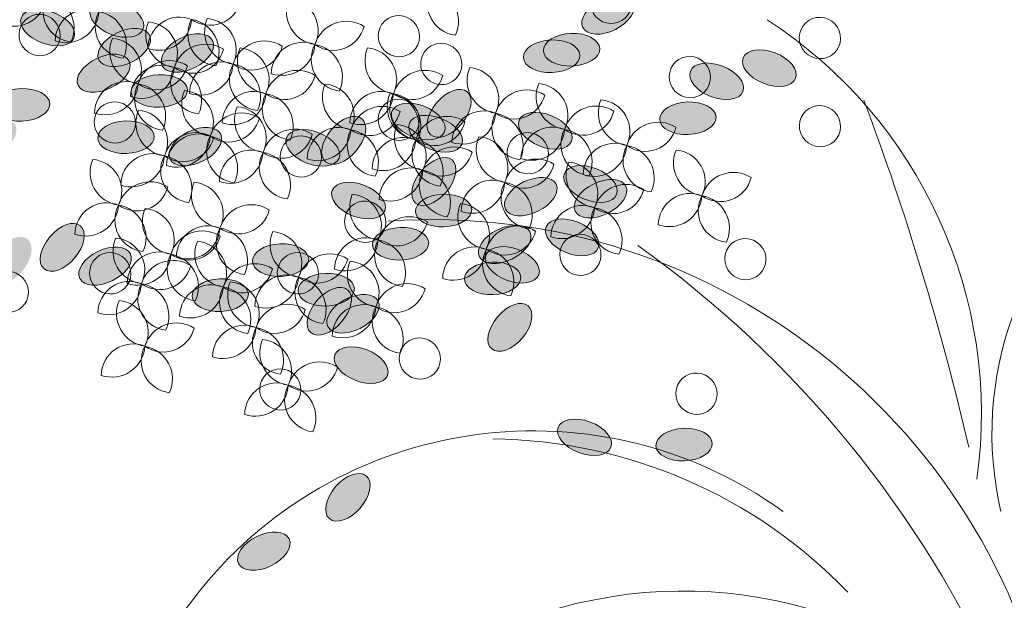
# Model space of a CAD drawing. Units: millimetres. Extents: x 595116 to 630915, y 909473 to 920225.
# Tile 13 of 134: x 629511 to 629534, y 919176 to 919190. Entities that reach past the tile are written whole.
import ezdxf

# ---------------------------------------------------------------- set-up
doc = ezdxf.new("R2010")
doc.units = ezdxf.units.MM
doc.layers.add('Dimension', color=3, linetype='Continuous', lineweight=18)
doc.layers.add('L-PLNT', color=85, linetype='Continuous', lineweight=13)
doc.styles.get("Standard").update_dxf_attribs({"font": 'arial.ttf'})
doc.dimstyles.new('ISO-25', dxfattribs={"dimtxt": 9, "dimasz": 6, "dimexe": 1.25, "dimexo": 0.625, "dimtad": 1, "dimlunit": 4, "dimtxsty": 'Standard', "dimcen": 2.5, "dimadec": 0, "dimazin": 0, "dimtfac": 1, "dimtmove": 0, "dimatfit": 3, "dimfxl": 1, "dimarcsym": 0})

# ---------------------------------------------------------------- blocks, each defined once
blk = doc.blocks.new('tree')
for centre, radius, start, end in [((629595.141, 919296.95), 5.184, 352.032, 57.0714), ((629604.232, 919296.737), 3.791, 61.1347, 193.108), ((629569.835, 919289.496), 31.168, 13.149, 20.5076), ((629594.259, 919292.132), 6.965, 7.4001, 94.0059), ((629589.446, 919288.922), 12.167, 24.2477, 54.3726), ((629595.377, 919292.044), 4.722, 54.2484, 144.2167), ((629594.88, 919291.171), 5.506, 43.8672, 89.4805), ((629597.025, 919289.989), 5.01, 36.0581, 170.6542)]:
    blk.add_arc(centre, radius, start, end)
blk = doc.blocks.new('A$C77972600')
h = blk.add_hatch(color=256)
edge = h.paths.add_edge_path()
edge.add_ellipse((3.0705, 5.8276), major_axis=(-0.1731, 0.0699), ratio=0.578492, start_angle=0, end_angle=360)
edge = h.paths.add_edge_path()
edge.add_ellipse((4.0989, 6.0027), major_axis=(-0.1319, 0.1321), ratio=0.578492, start_angle=0, end_angle=360)
edge = h.paths.add_edge_path()
edge.add_ellipse((4.5318, 6.7683), major_axis=(-0.1688, -0.0798), ratio=0.578492, start_angle=0, end_angle=360)
edge = h.paths.add_edge_path()
edge.add_ellipse((5.185, 6.8705), major_axis=(-0.1865, -0.0073), ratio=0.578492, start_angle=0, end_angle=360)
edge = h.paths.add_edge_path()
edge.add_ellipse((4.6885, 3.4464), major_axis=(-0.1865, -0.0073), ratio=0.578492, start_angle=0, end_angle=360)
edge = h.paths.add_edge_path()
edge.add_ellipse((4.5217, 4.2367), major_axis=(-0.1865, -0.0073), ratio=0.578492, start_angle=0, end_angle=360)
edge = h.paths.add_edge_path()
edge.add_ellipse((4.9166, 3.9946), major_axis=(-0.1731, 0.0699), ratio=0.578492, start_angle=0, end_angle=360)
edge = h.paths.add_edge_path()
edge.add_ellipse((3.6759, 4.9988), major_axis=(-0.1319, 0.1321), ratio=0.578492, start_angle=0, end_angle=360)
edge = h.paths.add_edge_path()
edge.add_ellipse((3.1035, 4.6784), major_axis=(-0.1319, 0.1321), ratio=0.578492, start_angle=0, end_angle=360)
edge = h.paths.add_edge_path()
edge.add_ellipse((3.8133, 4.5577), major_axis=(-0.1319, 0.1321), ratio=0.578492, start_angle=0, end_angle=360)
edge = h.paths.add_edge_path()
edge.add_ellipse((2.2042, 5.6327), major_axis=(-0.1865, -0.0073), ratio=0.578492, start_angle=0, end_angle=360)
edge = h.paths.add_edge_path()
edge.add_ellipse((2.9066, 5.6543), major_axis=(-0.1865, -0.0073), ratio=0.578492, start_angle=0, end_angle=360)
edge = h.paths.add_edge_path()
edge.add_ellipse((2.6215, 5.4344), major_axis=(-0.1865, -0.0073), ratio=0.578492, start_angle=0, end_angle=360)
edge = h.paths.add_edge_path()
edge.add_ellipse((2.1195, 4.0174), major_axis=(-0.1731, 0.0699), ratio=0.578492, start_angle=0, end_angle=360)
edge = h.paths.add_edge_path()
edge.add_ellipse((4.1491, 5.5914), major_axis=(-0.1688, -0.0798), ratio=0.578492, start_angle=0, end_angle=360)
edge = h.paths.add_edge_path()
edge.add_ellipse((1.9571, 3.173), major_axis=(-0.1865, -0.0073), ratio=0.578492, start_angle=0, end_angle=360)
edge = h.paths.add_edge_path()
edge.add_ellipse((1.589, 3.2907), major_axis=(-0.1688, -0.0798), ratio=0.578492, start_angle=0, end_angle=360)
edge = h.paths.add_edge_path()
edge.add_ellipse((1.045, 3.0811), major_axis=(-0.1865, -0.0073), ratio=0.578492, start_angle=0, end_angle=360)
edge = h.paths.add_edge_path()
edge.add_ellipse((1.2104, 3.7739), major_axis=(-0.1688, -0.0798), ratio=0.578492, start_angle=0, end_angle=360)
edge = h.paths.add_edge_path()
edge.add_ellipse((1.6721, 3.755), major_axis=(-0.1688, -0.0798), ratio=0.578492, start_angle=0, end_angle=360)
edge = h.paths.add_edge_path()
edge.add_ellipse((0.772, 4.473), major_axis=(-0.1731, 0.0699), ratio=0.578492, start_angle=0, end_angle=360)
edge = h.paths.add_edge_path()
edge.add_ellipse((0.8326, 5.2916), major_axis=(-0.1319, 0.1321), ratio=0.578492, start_angle=0, end_angle=360)
edge = h.paths.add_edge_path()
edge.add_ellipse((1.1875, 5.2313), major_axis=(-0.1319, 0.1321), ratio=0.578492, start_angle=0, end_angle=360)
edge = h.paths.add_edge_path()
edge.add_ellipse((5.3876, 4.7197), major_axis=(-0.1865, -0.0073), ratio=0.578492, start_angle=0, end_angle=360)
edge = h.paths.add_edge_path()
edge.add_ellipse((3.5552, 2.162), major_axis=(-0.1865, -0.0073), ratio=0.578492, start_angle=0, end_angle=360)
edge = h.paths.add_edge_path()
edge.add_ellipse((3.8402, 2.3819), major_axis=(-0.1865, -0.0073), ratio=0.578492, start_angle=0, end_angle=360)
edge = h.paths.add_edge_path()
edge.add_ellipse((4.692, 2.204), major_axis=(-0.1731, 0.0699), ratio=0.578492, start_angle=0, end_angle=360)
edge = h.paths.add_edge_path()
edge.add_ellipse((4.514, 2.9096), major_axis=(-0.1731, 0.0699), ratio=0.578492, start_angle=0, end_angle=360)
edge = h.paths.add_edge_path()
edge.add_ellipse((4.8133, 2.5575), major_axis=(-0.1731, 0.0699), ratio=0.578492, start_angle=0, end_angle=360)
edge = h.paths.add_edge_path()
edge.add_ellipse((3.7876, 2.8899), major_axis=(-0.1731, 0.0699), ratio=0.578492, start_angle=0, end_angle=360)
h = blk.add_hatch(color=256)
edge = h.paths.add_edge_path()
edge.add_ellipse((3.2403, 1.6985), major_axis=(-0.1668, -0.0838), ratio=0.578492, start_angle=0, end_angle=360, ccw=False)
edge = h.paths.add_edge_path()
edge.add_ellipse((4.2796, 1.6084), major_axis=(-0.1206, -0.1425), ratio=0.578492, start_angle=0, end_angle=360, ccw=False)
edge = h.paths.add_edge_path()
edge.add_ellipse((4.7739, 0.881), major_axis=(-0.1747, 0.0657), ratio=0.578492, start_angle=0, end_angle=360, ccw=False)
edge = h.paths.add_edge_path()
edge.add_ellipse((5.4333, 0.8328), major_axis=(-0.1865, -0.008), ratio=0.578492, start_angle=0, end_angle=360, ccw=False)
edge = h.paths.add_edge_path()
edge.add_ellipse((4.6573, 4.2045), major_axis=(-0.1865, -0.008), ratio=0.578492, start_angle=0, end_angle=360, ccw=False)
edge = h.paths.add_edge_path()
edge.add_ellipse((4.556, 3.4032), major_axis=(-0.1865, -0.008), ratio=0.578492, start_angle=0, end_angle=360, ccw=False)
edge = h.paths.add_edge_path()
edge.add_ellipse((4.9297, 3.677), major_axis=(-0.1668, -0.0838), ratio=0.578492, start_angle=0, end_angle=360, ccw=False)
edge = h.paths.add_edge_path()
edge.add_ellipse((3.7756, 2.5742), major_axis=(-0.1206, -0.1425), ratio=0.578492, start_angle=0, end_angle=360, ccw=False)
edge = h.paths.add_edge_path()
edge.add_ellipse((3.1788, 2.8466), major_axis=(-0.1206, -0.1425), ratio=0.578492, start_angle=0, end_angle=360, ccw=False)
edge = h.paths.add_edge_path()
edge.add_ellipse((3.8763, 3.0252), major_axis=(-0.1206, -0.1425), ratio=0.578492, start_angle=0, end_angle=360, ccw=False)
edge = h.paths.add_edge_path()
edge.add_ellipse((2.3609, 1.8217), major_axis=(-0.1865, -0.008), ratio=0.578492, start_angle=0, end_angle=360, ccw=False)
edge = h.paths.add_edge_path()
edge.add_ellipse((3.0627, 1.8578), major_axis=(-0.1865, -0.008), ratio=0.578492, start_angle=0, end_angle=360, ccw=False)
edge = h.paths.add_edge_path()
edge.add_ellipse((2.7605, 2.0535), major_axis=(-0.1865, -0.008), ratio=0.578492, start_angle=0, end_angle=360, ccw=False)
edge = h.paths.add_edge_path()
edge.add_ellipse((2.1439, 3.4246), major_axis=(-0.1668, -0.0838), ratio=0.578492, start_angle=0, end_angle=360, ccw=False)
edge = h.paths.add_edge_path()
edge.add_ellipse((4.2959, 2.0225), major_axis=(-0.1747, 0.0657), ratio=0.578492, start_angle=0, end_angle=360, ccw=False)
edge = h.paths.add_edge_path()
edge.add_ellipse((1.9127, 4.2528), major_axis=(-0.1865, -0.008), ratio=0.578492, start_angle=0, end_angle=360, ccw=False)
edge = h.paths.add_edge_path()
edge.add_ellipse((1.5555, 4.1052), major_axis=(-0.1747, 0.0657), ratio=0.578492, start_angle=0, end_angle=360, ccw=False)
edge = h.paths.add_edge_path()
edge.add_ellipse((0.9962, 4.2695), major_axis=(-0.1865, -0.008), ratio=0.578492, start_angle=0, end_angle=360, ccw=False)
edge = h.paths.add_edge_path()
edge.add_ellipse((1.2179, 3.5926), major_axis=(-0.1747, 0.0657), ratio=0.578492, start_angle=0, end_angle=360, ccw=False)
edge = h.paths.add_edge_path()
edge.add_ellipse((1.6764, 3.6493), major_axis=(-0.1747, 0.0657), ratio=0.578492, start_angle=0, end_angle=360, ccw=False)
edge = h.paths.add_edge_path()
edge.add_ellipse((0.8384, 2.8599), major_axis=(-0.1668, -0.0838), ratio=0.578492, start_angle=0, end_angle=360, ccw=False)
edge = h.paths.add_edge_path()
edge.add_ellipse((0.9659, 2.049), major_axis=(-0.1206, -0.1425), ratio=0.578492, start_angle=0, end_angle=360, ccw=False)
edge = h.paths.add_edge_path()
edge.add_ellipse((1.3147, 2.1383), major_axis=(-0.1206, -0.1425), ratio=0.578492, start_angle=0, end_angle=360, ccw=False)
edge = h.paths.add_edge_path()
edge.add_ellipse((5.4586, 2.9929), major_axis=(-0.1865, -0.008), ratio=0.578492, start_angle=0, end_angle=360, ccw=False)
edge = h.paths.add_edge_path()
edge.add_ellipse((3.4224, 5.3915), major_axis=(-0.1865, -0.008), ratio=0.578492, start_angle=0, end_angle=360, ccw=False)
edge = h.paths.add_edge_path()
edge.add_ellipse((3.7245, 5.1958), major_axis=(-0.1865, -0.008), ratio=0.578492, start_angle=0, end_angle=360, ccw=False)
edge = h.paths.add_edge_path()
edge.add_ellipse((4.5588, 5.4431), major_axis=(-0.1668, -0.0838), ratio=0.578492, start_angle=0, end_angle=360, ccw=False)
edge = h.paths.add_edge_path()
edge.add_ellipse((4.4393, 4.7252), major_axis=(-0.1668, -0.0838), ratio=0.578492, start_angle=0, end_angle=360, ccw=False)
edge = h.paths.add_edge_path()
edge.add_ellipse((4.7087, 5.1006), major_axis=(-0.1668, -0.0838), ratio=0.578492, start_angle=0, end_angle=360, ccw=False)
edge = h.paths.add_edge_path()
edge.add_ellipse((3.7138, 4.6852), major_axis=(-0.1668, -0.0838), ratio=0.578492, start_angle=0, end_angle=360, ccw=False)
h = blk.add_hatch(color=256)
edge = h.paths.add_edge_path()
edge.add_ellipse((4.1652, 1.933), major_axis=(0.1866, 0.0058), ratio=0.578492, start_angle=0, end_angle=360)
edge = h.paths.add_edge_path()
edge.add_ellipse((3.2944, 1.3586), major_axis=(0.1739, -0.0678), ratio=0.578492, start_angle=0, end_angle=360)
edge = h.paths.add_edge_path()
edge.add_ellipse((3.2064, 0.4835), major_axis=(0.1223, 0.141), ratio=0.578492, start_angle=0, end_angle=360)
edge = h.paths.add_edge_path()
edge.add_ellipse((2.6497, 0.127), major_axis=(0.1678, 0.0818), ratio=0.578492, start_angle=0, end_angle=360)
edge = h.paths.add_edge_path()
edge.add_ellipse((1.7252, 3.461), major_axis=(0.1678, 0.0818), ratio=0.578492, start_angle=0, end_angle=360)
edge = h.paths.add_edge_path()
edge.add_ellipse((2.1962, 2.8048), major_axis=(0.1678, 0.0818), ratio=0.578492, start_angle=0, end_angle=360)
edge = h.paths.add_edge_path()
edge.add_ellipse((1.7372, 2.8674), major_axis=(0.1866, 0.0058), ratio=0.578492, start_angle=0, end_angle=360)
edge = h.paths.add_edge_path()
edge.add_ellipse((3.2773, 2.4479), major_axis=(0.1739, -0.0678), ratio=0.578492, start_angle=0, end_angle=360)
edge = h.paths.add_edge_path()
edge.add_ellipse((3.6722, 2.9717), major_axis=(0.1739, -0.0678), ratio=0.578492, start_angle=0, end_angle=360)
edge = h.paths.add_edge_path()
edge.add_ellipse((2.9739, 2.7963), major_axis=(0.1739, -0.0678), ratio=0.578492, start_angle=0, end_angle=360)
edge = h.paths.add_edge_path()
edge.add_ellipse((4.8796, 2.4604), major_axis=(0.1678, 0.0818), ratio=0.578492, start_angle=0, end_angle=360)
edge = h.paths.add_edge_path()
edge.add_ellipse((4.2454, 2.1577), major_axis=(0.1678, 0.0818), ratio=0.578492, start_angle=0, end_angle=360)
edge = h.paths.add_edge_path()
edge.add_ellipse((4.4178, 2.4738), major_axis=(0.1678, 0.0818), ratio=0.578492, start_angle=0, end_angle=360)
edge = h.paths.add_edge_path()
edge.add_ellipse((4.3066, 3.973), major_axis=(0.1866, 0.0058), ratio=0.578492, start_angle=0, end_angle=360)
edge = h.paths.add_edge_path()
edge.add_ellipse((3.0828, 1.7149), major_axis=(0.1223, 0.141), ratio=0.578492, start_angle=0, end_angle=360)
edge = h.paths.add_edge_path()
edge.add_ellipse((4.1152, 4.8113), major_axis=(0.1678, 0.0818), ratio=0.578492, start_angle=0, end_angle=360)
edge = h.paths.add_edge_path()
edge.add_ellipse((4.4995, 4.8518), major_axis=(0.1223, 0.141), ratio=0.578492, start_angle=0, end_angle=360)
edge = h.paths.add_edge_path()
edge.add_ellipse((4.913, 5.2627), major_axis=(0.1678, 0.0818), ratio=0.578492, start_angle=0, end_angle=360)
edge = h.paths.add_edge_path()
edge.add_ellipse((5.0407, 4.562), major_axis=(0.1223, 0.141), ratio=0.578492, start_angle=0, end_angle=360)
edge = h.paths.add_edge_path()
edge.add_ellipse((4.6105, 4.3933), major_axis=(0.1223, 0.141), ratio=0.578492, start_angle=0, end_angle=360)
edge = h.paths.add_edge_path()
edge.add_ellipse((5.7235, 4.0986), major_axis=(0.1866, 0.0058), ratio=0.578492, start_angle=0, end_angle=360)
edge = h.paths.add_edge_path()
edge.add_ellipse((5.9977, 3.3249), major_axis=(0.1739, -0.0678), ratio=0.578492, start_angle=0, end_angle=360)
edge = h.paths.add_edge_path()
edge.add_ellipse((5.6486, 3.2372), major_axis=(0.1739, -0.0678), ratio=0.578492, start_angle=0, end_angle=360)
edge = h.paths.add_edge_path()
edge.add_ellipse((1.5981, 2.014), major_axis=(0.1678, 0.0818), ratio=0.578492, start_angle=0, end_angle=360)
edge = h.paths.add_edge_path()
edge.add_ellipse((2.2453, 5.0931), major_axis=(0.1678, 0.0818), ratio=0.578492, start_angle=0, end_angle=360)
edge = h.paths.add_edge_path()
edge.add_ellipse((2.073, 4.777), major_axis=(0.1678, 0.0818), ratio=0.578492, start_angle=0, end_angle=360)
edge = h.paths.add_edge_path()
edge.add_ellipse((1.2216, 4.5968), major_axis=(0.1866, 0.0058), ratio=0.578492, start_angle=0, end_angle=360)
edge = h.paths.add_edge_path()
edge.add_ellipse((1.6688, 4.0227), major_axis=(0.1866, 0.0058), ratio=0.578492, start_angle=0, end_angle=360)
edge = h.paths.add_edge_path()
edge.add_ellipse((1.253, 4.2244), major_axis=(0.1866, 0.0058), ratio=0.578492, start_angle=0, end_angle=360)
edge = h.paths.add_edge_path()
edge.add_ellipse((2.3257, 4.3332), major_axis=(0.1866, 0.0058), ratio=0.578492, start_angle=0, end_angle=360)
for centre, radius, start, end in [((3.9437, 3.7517), 0.2106, 152.13841, 263.31486), ((3.721, 3.6346), 0.2185, 335.05813, 80.39514), ((1.1322, 3.6106), 0.2106, 68.14697, 179.32342), ((0.9925, 3.8198), 0.2185, 251.0667, 356.4037), ((1.3968, 3.7077), 0.2106, 152.13841, 263.31486), ((1.1741, 3.5907), 0.2185, 335.05813, 80.39514), ((3.0179, 3.6973), 0.2185, 156.8071, 262.14411), ((2.7989, 3.5735), 0.2106, 333.88738, 85.06383), ((2.2928, 3.8191), 0.2106, 234.66708, 345.84353), ((1.479, 3.5022), 0.2106, 68.14697, 179.32342), ((1.3393, 3.7114), 0.2185, 251.0667, 356.4037), ((1.7436, 3.5992), 0.2106, 152.13841, 263.31486), ((1.5209, 3.4822), 0.2185, 335.05813, 80.39514), ((2.0926, 3.4517), 0.2106, 68.14697, 179.32342), ((2.476, 3.5671), 0.2185, 156.8071, 262.14411), ((2.257, 3.4433), 0.2106, 333.88738, 85.06383), ((2.0858, 3.5454), 0.2185, 156.8071, 262.14411), ((1.9529, 3.6609), 0.2185, 251.0667, 356.4037), ((1.8668, 3.4216), 0.2106, 333.88738, 85.06383), ((2.3572, 3.5488), 0.2106, 152.13841, 263.31486), ((2.1345, 3.4318), 0.2185, 335.05813, 80.39514), ((3.1969, 3.4166), 0.2185, 57.5868, 162.92381), ((3.1098, 3.6526), 0.2106, 234.66708, 345.84353), ((1.8474, 3.437), 0.2185, 156.8071, 262.14411), ((1.6284, 3.3132), 0.2106, 333.88738, 85.06383), ((2.2649, 3.2648), 0.2185, 57.5868, 162.92381), ((2.655, 3.2865), 0.2185, 57.5868, 162.92381), ((2.5679, 3.5225), 0.2106, 234.66708, 345.84353), ((2.6928, 3.3719), 0.2185, 156.8071, 262.14411), ((2.4738, 3.2481), 0.2106, 333.88738, 85.06383), ((2.9096, 3.2853), 0.2106, 68.14697, 179.32342), ((2.7699, 3.4945), 0.2185, 251.0667, 356.4037), ((3.1742, 3.3823), 0.2106, 152.13841, 263.31486), ((2.9516, 3.2653), 0.2185, 335.05813, 80.39514), ((3.5381, 3.3719), 0.2185, 156.8071, 262.14411), ((3.3191, 3.2481), 0.2106, 333.88738, 85.06383), ((2.1778, 3.5008), 0.2106, 234.66708, 345.84353), ((1.9776, 3.1335), 0.2106, 68.14697, 179.32342), ((1.8379, 3.3427), 0.2185, 251.0667, 356.4037), ((2.0264, 3.1563), 0.2185, 57.5868, 162.92381), ((1.9393, 3.3923), 0.2106, 234.66708, 345.84353), ((2.2422, 3.2305), 0.2106, 152.13841, 263.31486), ((2.0195, 3.1135), 0.2185, 335.05813, 80.39514), ((2.3677, 3.1551), 0.2106, 68.14697, 179.32342), ((2.228, 3.3643), 0.2185, 251.0667, 356.4037), ((2.6323, 3.2522), 0.2106, 152.13841, 263.31486), ((2.4097, 3.1352), 0.2185, 335.05813, 80.39514), ((4.2143, 3.2426), 0.2185, 156.8071, 262.14411), ((3.9953, 3.1188), 0.2106, 333.88738, 85.06383), ((2.8718, 3.0912), 0.2185, 57.5868, 162.92381), ((2.7847, 3.3273), 0.2106, 234.66708, 345.84353), ((3.7172, 3.0912), 0.2185, 57.5868, 162.92381), ((3.6301, 3.3273), 0.2106, 234.66708, 345.84353), ((1.7391, 3.025), 0.2106, 68.14697, 179.32342), ((1.5994, 3.2342), 0.2185, 251.0667, 356.4037), ((2.0037, 3.1221), 0.2106, 152.13841, 263.31486), ((1.7811, 3.005), 0.2185, 335.05813, 80.39514), ((3.2563, 3.1333), 0.2185, 156.8071, 262.14411), ((3.0373, 3.0095), 0.2106, 333.88738, 85.06383), ((4.6718, 3.1358), 0.2185, 156.8071, 262.14411), ((4.4528, 3.012), 0.2106, 333.88738, 85.06383), ((2.3243, 3.0899), 0.2185, 156.8071, 262.14411), ((2.1053, 2.9661), 0.2106, 333.88738, 85.06383), ((2.5845, 2.9599), 0.2106, 68.14697, 179.32342), ((2.4448, 3.1691), 0.2185, 251.0667, 356.4037), ((2.8491, 3.057), 0.2106, 152.13841, 263.31486), ((2.6264, 2.9399), 0.2185, 335.05813, 80.39514), ((3.4299, 2.9599), 0.2106, 68.14697, 179.32342), ((3.2902, 3.1691), 0.2185, 251.0667, 356.4037), ((3.6857, 3.0673), 0.2185, 156.8071, 262.14411), ((3.6945, 3.057), 0.2106, 152.13841, 263.31486), ((3.4667, 2.9435), 0.2106, 333.88738, 85.06383), ((3.4718, 2.9399), 0.2185, 335.05813, 80.39514), ((4.3933, 2.9619), 0.2185, 57.5868, 162.92381), ((4.3062, 3.1979), 0.2106, 234.66708, 345.84353), ((2.6742, 2.9832), 0.2185, 156.8071, 262.14411), ((2.4552, 2.8594), 0.2106, 333.88738, 85.06383), ((3.4354, 2.8527), 0.2185, 57.5868, 162.92381), ((4.8508, 2.8551), 0.2185, 57.5868, 162.92381), ((5.0835, 3.029), 0.2185, 156.8071, 262.14411), ((4.8645, 2.9052), 0.2106, 333.88738, 85.06383), ((2.0208, 2.9598), 0.2185, 156.8071, 262.14411), ((1.8018, 2.836), 0.2106, 333.88738, 85.06383), ((2.5033, 2.8093), 0.2185, 57.5868, 162.92381), ((3.3483, 3.0887), 0.2106, 234.66708, 345.84353), ((3.8647, 2.7867), 0.2185, 57.5868, 162.92381), ((4.106, 2.8306), 0.2106, 68.14697, 179.32342), ((3.9663, 3.0398), 0.2185, 251.0667, 356.4037), ((4.3707, 2.9277), 0.2106, 152.13841, 263.31486), ((4.148, 2.8106), 0.2185, 335.05813, 80.39514), ((4.7637, 3.0911), 0.2106, 234.66708, 345.84353), ((2.4162, 3.0453), 0.2106, 234.66708, 345.84353), ((3.7332, 2.8653), 0.2185, 156.8071, 262.14411), ((3.5142, 2.7415), 0.2106, 333.88738, 85.06383), ((3.7776, 3.0227), 0.2106, 234.66708, 345.84353), ((5.2625, 2.7483), 0.2185, 57.5868, 162.92381), ((2.1998, 2.6791), 0.2185, 57.5868, 162.92381), ((2.216, 2.678), 0.2106, 68.14697, 179.32342), ((2.0763, 2.8872), 0.2185, 251.0667, 356.4037), ((2.4806, 2.775), 0.2106, 152.13841, 263.31486), ((2.2579, 2.658), 0.2185, 335.05813, 80.39514), ((2.8532, 2.7025), 0.2185, 57.5868, 162.92381), ((2.7661, 2.9385), 0.2106, 234.66708, 345.84353), ((3.1481, 2.7213), 0.2106, 68.14697, 179.32342), ((3.0084, 2.9305), 0.2185, 251.0667, 356.4037), ((3.4127, 2.8184), 0.2106, 152.13841, 263.31486), ((3.19, 2.7014), 0.2185, 335.05813, 80.39514), ((4.2753, 2.7848), 0.2185, 156.8071, 262.14411), ((4.0563, 2.661), 0.2106, 333.88738, 85.06383), ((4.5635, 2.7238), 0.2106, 68.14697, 179.32342), ((4.4238, 2.933), 0.2185, 251.0667, 356.4037), ((4.8281, 2.8208), 0.2106, 152.13841, 263.31486), ((4.6054, 2.7038), 0.2185, 335.05813, 80.39514), ((5.1754, 2.9843), 0.2106, 234.66708, 345.84353), ((2.1127, 2.9151), 0.2106, 234.66708, 345.84353), ((3.5774, 2.6553), 0.2106, 68.14697, 179.32342), ((3.4377, 2.8645), 0.2185, 251.0667, 356.4037), ((3.842, 2.7524), 0.2106, 152.13841, 263.31486), ((3.6193, 2.6354), 0.2185, 335.05813, 80.39514), ((4.9752, 2.617), 0.2106, 68.14697, 179.32342), ((4.8355, 2.8262), 0.2185, 251.0667, 356.4037), ((5.2398, 2.714), 0.2106, 152.13841, 263.31486), ((5.0172, 2.597), 0.2185, 335.05813, 80.39514), ((1.9125, 2.5478), 0.2106, 68.14697, 179.32342), ((1.7728, 2.757), 0.2185, 251.0667, 356.4037), ((2.1771, 2.6449), 0.2106, 152.13841, 263.31486), ((1.9545, 2.5278), 0.2185, 335.05813, 80.39514), ((2.5659, 2.5712), 0.2106, 68.14697, 179.32342), ((2.4262, 2.7804), 0.2185, 251.0667, 356.4037), ((2.8305, 2.6683), 0.2106, 152.13841, 263.31486), ((2.6078, 2.5512), 0.2185, 335.05813, 80.39514), ((3.9122, 2.5846), 0.2185, 57.5868, 162.92381), ((3.8251, 2.8206), 0.2106, 234.66708, 345.84353), ((5.5815, 2.6965), 0.2185, 156.8071, 262.14411), ((5.3625, 2.5727), 0.2106, 333.88738, 85.06383), ((1.7173, 2.6344), 0.2185, 156.8071, 262.14411), ((1.4983, 2.5106), 0.2106, 333.88738, 85.06383), ((4.4543, 2.5042), 0.2185, 57.5868, 162.92381), ((4.3672, 2.7402), 0.2106, 234.66708, 345.84353), ((4.87, 2.617), 0.2185, 156.8071, 262.14411), ((4.651, 2.4932), 0.2106, 333.88738, 85.06383), ((3.6249, 2.4533), 0.2106, 68.14697, 179.32342), ((3.4852, 2.6625), 0.2185, 251.0667, 356.4037), ((3.8895, 2.5503), 0.2106, 152.13841, 263.31486), ((3.6669, 2.4333), 0.2185, 335.05813, 80.39514), ((5.7605, 2.4158), 0.2185, 57.5868, 162.92381), ((1.8964, 2.3538), 0.2185, 57.5868, 162.92381), ((2.3893, 2.4826), 0.2185, 156.8071, 262.14411), ((2.1703, 2.3588), 0.2106, 333.88738, 85.06383), ((4.167, 2.3728), 0.2106, 68.14697, 179.32342), ((4.0273, 2.582), 0.2185, 251.0667, 356.4037), ((4.4316, 2.4699), 0.2106, 152.13841, 263.31486), ((4.209, 2.3529), 0.2185, 335.05813, 80.39514), ((5.049, 2.3363), 0.2185, 57.5868, 162.92381), ((5.6734, 2.6518), 0.2106, 234.66708, 345.84353), ((1.8093, 2.5898), 0.2106, 234.66708, 345.84353), ((3.4366, 2.4033), 0.2185, 156.8071, 262.14411), ((3.2176, 2.2796), 0.2106, 333.88738, 85.06383), ((4.962, 2.5723), 0.2106, 234.66708, 345.84353), ((5.4732, 2.2845), 0.2106, 68.14697, 179.32342), ((5.3335, 2.4937), 0.2185, 251.0667, 356.4037), ((5.7378, 2.3816), 0.2106, 152.13841, 263.31486), ((5.5151, 2.2645), 0.2185, 335.05813, 80.39514), ((1.6091, 2.2224), 0.2106, 68.14697, 179.32342), ((1.4694, 2.4316), 0.2185, 251.0667, 356.4037), ((1.8737, 2.3195), 0.2106, 152.13841, 263.31486), ((1.651, 2.2025), 0.2185, 335.05813, 80.39514), ((2.5683, 2.2019), 0.2185, 57.5868, 162.92381), ((4.1533, 2.3423), 0.2185, 156.8071, 262.14411), ((3.9343, 2.2185), 0.2106, 333.88738, 85.06383), ((4.7617, 2.205), 0.2106, 68.14697, 179.32342), ((2.0642, 2.3091), 0.2185, 156.8071, 262.14411), ((1.8452, 2.1853), 0.2106, 333.88738, 85.06383), ((2.4812, 2.4379), 0.2106, 234.66708, 345.84353), ((4.622, 2.4142), 0.2185, 251.0667, 356.4037), ((5.0264, 2.302), 0.2106, 152.13841, 263.31486), ((4.8037, 2.185), 0.2185, 335.05813, 80.39514), ((3.6156, 2.1227), 0.2185, 57.5868, 162.92381), ((3.5286, 2.3587), 0.2106, 234.66708, 345.84353), ((2.2432, 2.0284), 0.2185, 57.5868, 162.92381), ((2.281, 2.0706), 0.2106, 68.14697, 179.32342), ((2.1413, 2.2798), 0.2185, 251.0667, 356.4037), ((2.5456, 2.1677), 0.2106, 152.13841, 263.31486), ((2.323, 2.0506), 0.2185, 335.05813, 80.39514), ((2.9095, 2.1572), 0.2185, 156.8071, 262.14411), ((2.6905, 2.0335), 0.2106, 333.88738, 85.06383), ((4.3323, 2.0616), 0.2185, 57.5868, 162.92381), ((4.2453, 2.2976), 0.2106, 234.66708, 345.84353), ((1.8691, 2.1139), 0.2185, 156.8071, 262.14411), ((1.6501, 1.9901), 0.2106, 333.88738, 85.06383), ((2.1561, 2.2644), 0.2106, 234.66708, 345.84353), ((2.411, 2.0922), 0.2185, 156.8071, 262.14411), ((2.192, 1.9684), 0.2106, 333.88738, 85.06383), ((3.3283, 1.9914), 0.2106, 68.14697, 179.32342), ((3.1886, 2.2006), 0.2185, 251.0667, 356.4037), ((3.593, 2.0884), 0.2106, 152.13841, 263.31486), ((3.3703, 1.9714), 0.2185, 335.05813, 80.39514), ((1.9559, 1.8971), 0.2106, 68.14697, 179.32342), ((1.8162, 2.1063), 0.2185, 251.0667, 356.4037), ((2.2205, 1.9941), 0.2106, 152.13841, 263.31486), ((1.9978, 1.8771), 0.2185, 335.05813, 80.39514), ((3.0886, 1.8766), 0.2185, 57.5868, 162.92381), ((4.045, 1.9303), 0.2106, 68.14697, 179.32342), ((3.9053, 2.1395), 0.2185, 251.0667, 356.4037), ((4.3097, 2.0274), 0.2106, 152.13841, 263.31486), ((4.087, 1.9103), 0.2185, 335.05813, 80.39514), ((2.0481, 1.8332), 0.2185, 57.5868, 162.92381), ((2.59, 1.8115), 0.2185, 57.5868, 162.92381), ((3.0015, 2.1126), 0.2106, 234.66708, 345.84353), ((3.4214, 1.9608), 0.2185, 156.8071, 262.14411), ((3.2024, 1.837), 0.2106, 333.88738, 85.06383), ((1.961, 2.0692), 0.2106, 234.66708, 345.84353), ((2.5029, 2.0475), 0.2106, 234.66708, 345.84353), ((1.7608, 1.7019), 0.2106, 68.14697, 179.32342), ((1.6211, 1.9111), 0.2185, 251.0667, 356.4037), ((2.0254, 1.7989), 0.2106, 152.13841, 263.31486), ((1.8027, 1.6819), 0.2185, 335.05813, 80.39514), ((2.6284, 1.8235), 0.2185, 156.8071, 262.14411), ((2.4094, 1.6997), 0.2106, 333.88738, 85.06383), ((2.8012, 1.7453), 0.2106, 68.14697, 179.32342), ((2.6615, 1.9545), 0.2185, 251.0667, 356.4037), ((3.0659, 1.8423), 0.2106, 152.13841, 263.31486), ((2.8432, 1.7253), 0.2185, 335.05813, 80.39514), ((3.6004, 1.6802), 0.2185, 57.5868, 162.92381), ((2.3027, 1.6802), 0.2106, 68.14697, 179.32342), ((2.163, 1.8894), 0.2185, 251.0667, 356.4037), ((2.5673, 1.7772), 0.2106, 152.13841, 263.31486), ((2.3446, 1.6602), 0.2185, 335.05813, 80.39514), ((3.5133, 1.9162), 0.2106, 234.66708, 345.84353), ((1.892, 1.7004), 0.2185, 156.8071, 262.14411), ((1.673, 1.5766), 0.2106, 333.88738, 85.06383), ((2.8075, 1.5428), 0.2185, 57.5868, 162.92381), ((2.7204, 1.7788), 0.2106, 234.66708, 345.84353), ((3.3131, 1.5488), 0.2106, 68.14697, 179.32342), ((3.1734, 1.758), 0.2185, 251.0667, 356.4037), ((3.5777, 1.6459), 0.2106, 152.13841, 263.31486), ((3.355, 1.5289), 0.2185, 335.05813, 80.39514), ((2.0711, 1.4197), 0.2185, 57.5868, 162.92381), ((1.984, 1.6557), 0.2106, 234.66708, 345.84353), ((2.5202, 1.4115), 0.2106, 68.14697, 179.32342), ((2.3804, 1.6207), 0.2185, 251.0667, 356.4037), ((2.7848, 1.5086), 0.2106, 152.13841, 263.31486), ((2.5621, 1.3915), 0.2185, 335.05813, 80.39514), ((2.8419, 1.442), 0.2185, 156.8071, 262.14411), ((2.6229, 1.3182), 0.2106, 333.88738, 85.06383), ((1.7838, 1.2884), 0.2106, 68.14697, 179.32342), ((1.644, 1.4976), 0.2185, 251.0667, 356.4037), ((2.0484, 1.3855), 0.2106, 152.13841, 263.31486), ((1.8257, 1.2684), 0.2185, 335.05813, 80.39514), ((3.0209, 1.1614), 0.2185, 57.5868, 162.92381), ((2.9338, 1.3974), 0.2106, 234.66708, 345.84353), ((2.7336, 1.03), 0.2106, 68.14697, 179.32342), ((2.5939, 1.2392), 0.2185, 251.0667, 356.4037), ((2.9982, 1.1271), 0.2106, 152.13841, 263.31486), ((2.7756, 1.0101), 0.2185, 335.05813, 80.39514)]:
    blk.add_arc(centre, radius, start, end)
for centre, major_axis, ratio in [((4.9485, 3.7567), (-0.0941, 0.1005), 0.985729), ((1.1648, 3.5436), (-0.0941, 0.1005), 0.985729), ((3.5445, 3.5362), (-0.0941, 0.1005), 0.985729), ((6.3331, 3.524), (-0.0941, 0.1005), 0.985729), ((3.8252, 3.3525), (-0.0941, 0.1005), 0.985729), ((1.589, 3.2907), (-0.1688, -0.0798), 0.578492), ((5.4715, 3.2652), (-0.0941, 0.1005), 0.985729), ((3.5436, 2.9827), (-0.0941, 0.1005), 0.985729), ((1.6631, 2.9649), (-0.0941, 0.1005), 0.985729), ((6.3334, 2.9404), (-0.0941, 0.1005), 0.985729), ((2.8954, 2.7399), (-0.0941, 0.1005), 0.985729), ((4.3981, 2.7613), (-0.0941, 0.1005), 0.985729), ((3.3212, 2.3078), (-0.0941, 0.1005), 0.985729), ((4.7463, 2.0884), (-0.0941, 0.1005), 0.985729), ((5.8392, 2.0603), (-0.0941, 0.1005), 0.985729), ((1.6324, 1.9666), (-0.0941, 0.1005), 0.985729), ((2.8755, 1.9668), (-0.0941, 0.1005), 0.985729), ((0.9537, 1.8437), (-0.0941, 0.1005), 0.985729), ((3.6829, 1.4023), (-0.0941, 0.1005), 0.985729), ((2.7589, 1.1975), (-0.0941, 0.1005), 0.985729), ((5.5155, 1.1693), (-0.0941, 0.1005), 0.985729)]:
    blk.add_ellipse(centre, major_axis=major_axis, ratio=ratio)
at = {"extrusion": (0, 0, -1)}
for centre, major_axis in [((1.6764, 3.6493), (-0.1747, 0.0657)), ((1.2179, 3.5926), (-0.1747, 0.0657)), ((3.8763, 3.0252), (-0.1206, -0.1425)), ((3.1788, 2.8466), (-0.1206, -0.1425)), ((3.7756, 2.5742), (-0.1206, -0.1425)), ((1.3147, 2.1383), (-0.1206, -0.1425)), ((4.2959, 2.0225), (-0.1747, 0.0657)), ((4.2796, 1.6084), (-0.1206, -0.1425)), ((4.7739, 0.881), (-0.1747, 0.0657))]:
    blk.add_ellipse(centre, major_axis=major_axis, ratio=0.578492, dxfattribs=at)
for centre, major_axis in [((4.9297, 3.677), (-0.1668, -0.0838)), ((2.1439, 3.4246), (-0.1668, -0.0838)), ((4.556, 3.4032), (-0.1865, -0.008)), ((5.4586, 2.9929), (-0.1865, -0.008)), ((2.7605, 2.0535), (-0.1865, -0.008)), ((3.0627, 1.8578), (-0.1865, -0.008)), ((2.3609, 1.8217), (-0.1865, -0.008)), ((3.2403, 1.6985), (-0.1668, -0.0838)), ((5.4333, 0.8328), (-0.1865, -0.008))]:
    blk.add_ellipse(centre, major_axis=major_axis, ratio=0.578492, start_param=3.141593, end_param=9.424778, dxfattribs=at)
for centre, major_axis, start_param, end_param in [((1.7252, 3.461), (-0.1678, -0.0818), 4.712389, 10.995574), ((4.6885, 3.4464), (-0.1865, -0.0073), 1.570796326803303, 7.853981633982889), ((5.9977, 3.3249), (-0.1739, 0.0678), 3.141593, 9.424778), ((5.6486, 3.2372), (-0.1739, 0.0678), 3.141593, 9.424778), ((1.9571, 3.173), (-0.1865, -0.0073), 1.5707963267791, 7.853981633958686), ((1.045, 3.0811), (-0.1865, -0.0073), 1.570796326824091, 7.853981634003678), ((3.6722, 2.9717), (-0.1739, 0.0678), 3.141593, 9.424778), ((3.7876, 2.8899), (-0.1731, 0.0699), 1.570796326789708, 7.853981633969294), ((4.514, 2.9096), (-0.1731, 0.0699), 1.570796326796475, 7.853981633976061), ((1.7372, 2.8674), (-0.1866, -0.0058), 4.712389, 10.995574), ((2.1962, 2.8048), (-0.1678, -0.0818), -1.570796, 4.712389), ((2.9739, 2.7963), (-0.1739, 0.0678), 3.141593, 9.424778), ((4.8133, 2.5575), (-0.1731, 0.0699), 1.570796326818409, 7.853981633997996), ((4.4178, 2.4738), (-0.1678, -0.0818), -1.570796, 4.712389), ((3.2773, 2.4479), (-0.1739, 0.0678), 3.141593, 9.424778), ((4.8796, 2.4604), (-0.1678, -0.0818), -1.570796, 4.712389), ((3.8402, 2.3819), (-0.1865, -0.0073), 1.570796326801151, 7.853981633980737), ((4.2454, 2.1577), (-0.1678, -0.0818), -1.570796, 4.712389), ((4.692, 2.204), (-0.1731, 0.0699), 1.570796326828346, 7.853981634007933), ((3.5552, 2.162), (-0.1865, -0.0073), 1.570796326801176, 7.853981633980762), ((1.5981, 2.014), (-0.1678, -0.0818), 4.712389, 10.995574), ((4.1652, 1.933), (-0.1866, -0.0058), -1.570796, 4.712389), ((3.0828, 1.7149), (-0.1223, -0.141), 3.141593, 9.424778), ((3.2944, 1.3586), (-0.1739, 0.0678), 3.141593, 9.424778), ((3.2064, 0.4835), (-0.1223, -0.141), 3.141593, 9.424778), ((2.6497, 0.127), (-0.1678, -0.0818), -1.570796, 4.712389)]:
    blk.add_ellipse(centre, major_axis=major_axis, ratio=0.578492, start_param=start_param, end_param=end_param)
blk = doc.blocks.new('*D216')
at = {"layer": 'Defpoints', "color": 0, "transparency": 16777216}
for p in [(629743.541, 919411.928), (629505.041, 919411.828), (629743.541, 918832.378)]:
    blk.add_point(p, dxfattribs=at)
at = {"layer": 'Dimension', "color": 0, "lineweight": -2, "transparency": 16777216}
for p, q in [((629743.541, 919411.303), (629743.541, 918831.128)), ((629505.041, 919411.203), (629505.041, 918831.128)), ((629511.041, 918832.378), (629737.541, 918832.378))]:
    blk.add_line(p, q, dxfattribs=at)
at = {"layer": 'Dimension', "color": 0, "transparency": 16777216}
for points in [[(629511.041, 918833.378), (629511.041, 918831.378), (629505.041, 918832.378)], [(629737.541, 918833.378), (629737.541, 918831.378), (629743.541, 918832.378)]]:
    blk.add_solid(points, dxfattribs=at)
at = {"layer": 'Dimension', "color": 0, "transparency": 16777216, "insert": (629624.291, 918837.656), "char_height": 9, "attachment_point": 5}
blk.add_mtext('19\'-10 1/2"', dxfattribs=at)

msp = doc.modelspace()

# ---------------------------------------------------------------- block references
at = {"layer": 'L-PLNT'}
for name, p, xscale, yscale, zscale in [('A$C77972600', (629507.679, 919176.974), 3.512546757812034, 3.512546757812034, 3.512546757812034), ('tree', (-697468.256, -1018411.841), 2.107689410566463, 2.107689410566463, 2.107689410566463)]:
    msp.add_blockref(name, p, dxfattribs=dict(at, xscale=xscale, yscale=yscale, zscale=zscale))

# ---------------------------------------------------------------- dimensions: what is measured, and where the dimension line sits
at = {"layer": 'Dimension'}
dim = msp.add_linear_dim(base=(629743.541, 918832.378), p1=(629505.041, 919411.828), p2=(629743.541, 919411.928), dimstyle='ISO-25', override={"dimdec": 1, "dimlfac": 1, "dimrnd": 0, "dimzin": 1, "dimdsep": 46, "dimlunit": 4, "dimfrac": 2}, dxfattribs=at)
dim.commit()
dim.dimension.update_dxf_attribs({"geometry": '*D216', "text_midpoint": (629624.291, 918837.656)})

doc.saveas('drawing.dxf')
